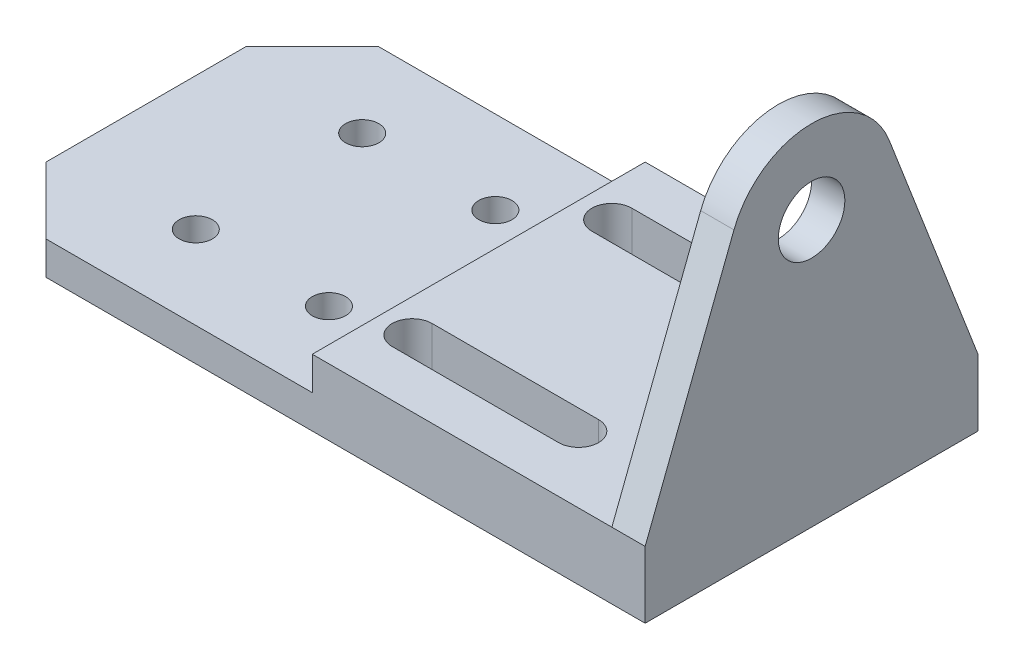
ISO-10303-21;
HEADER;
FILE_DESCRIPTION(('STEP AP214'),'2;1');
FILE_NAME('part.step','',(''),(''),'','','');
FILE_SCHEMA(('AUTOMOTIVE_DESIGN { 1 0 10303 214 1 1 1 1 }'));
ENDSEC;
DATA;
#1=APPLICATION_CONTEXT('core data for automotive mechanical design processes');
#2=APPLICATION_PROTOCOL_DEFINITION('international standard','automotive_design',2000,#1);
#3=PRODUCT_CONTEXT('',#1,'mechanical');
#4=PRODUCT('Part','Part','',(#3));
#5=PRODUCT_RELATED_PRODUCT_CATEGORY('part','',(#4));
#6=PRODUCT_DEFINITION_FORMATION('','',#4);
#7=PRODUCT_DEFINITION_CONTEXT('part definition',#1,'design');
#8=PRODUCT_DEFINITION('design','',#6,#7);
#9=PRODUCT_DEFINITION_SHAPE('','',#8);
#10=(LENGTH_UNIT() NAMED_UNIT(*) SI_UNIT(.MILLI.,.METRE.));
#11=(NAMED_UNIT(*) PLANE_ANGLE_UNIT() SI_UNIT($,.RADIAN.));
#12=(NAMED_UNIT(*) SI_UNIT($,.STERADIAN.) SOLID_ANGLE_UNIT());
#13=UNCERTAINTY_MEASURE_WITH_UNIT(LENGTH_MEASURE(1.E-05),#10,'distance_accuracy_value','');
#14=(GEOMETRIC_REPRESENTATION_CONTEXT(3) GLOBAL_UNCERTAINTY_ASSIGNED_CONTEXT((#13)) GLOBAL_UNIT_ASSIGNED_CONTEXT((#10,
#11,#12)) REPRESENTATION_CONTEXT('',''));
#15=CARTESIAN_POINT('',(0.,0.,0.));
#16=DIRECTION('',(0.,0.,1.));
#17=DIRECTION('',(1.,0.,0.));
#18=AXIS2_PLACEMENT_3D('',#15,#16,#17);
#19=CARTESIAN_POINT('',(0.,20.,100.));
#20=DIRECTION('',(1.,0.,0.));
#21=DIRECTION('',(0.,0.,-1.));
#22=AXIS2_PLACEMENT_3D('',#19,#20,#21);
#23=PLANE('',#22);
#24=DIRECTION('',(0.,0.,-1.));
#25=VECTOR('',#24,1.);
#26=CARTESIAN_POINT('',(0.,10.,100.));
#27=LINE('',#26,#25);
#28=CARTESIAN_POINT('',(0.,10.,100.));
#29=VERTEX_POINT('',#28);
#30=CARTESIAN_POINT('',(0.,10.,0.));
#31=VERTEX_POINT('',#30);
#32=EDGE_CURVE('E279',#29,#31,#27,.T.);
#33=ORIENTED_EDGE('',*,*,#32,.F.);
#34=DIRECTION('',(0.,-1.,0.));
#35=VECTOR('',#34,1.);
#36=CARTESIAN_POINT('',(0.,20.,100.));
#37=LINE('',#36,#35);
#38=CARTESIAN_POINT('',(0.,20.,100.));
#39=VERTEX_POINT('',#38);
#40=EDGE_CURVE('E295',#39,#29,#37,.T.);
#41=ORIENTED_EDGE('',*,*,#40,.F.);
#42=DIRECTION('',(0.,0.,-1.));
#43=VECTOR('',#42,1.);
#44=CARTESIAN_POINT('',(0.,20.,100.));
#45=LINE('',#44,#43);
#46=CARTESIAN_POINT('',(0.,20.,0.));
#47=VERTEX_POINT('',#46);
#48=EDGE_CURVE('E302',#39,#47,#45,.T.);
#49=ORIENTED_EDGE('',*,*,#48,.T.);
#50=DIRECTION('',(0.,-1.,0.));
#51=VECTOR('',#50,1.);
#52=CARTESIAN_POINT('',(0.,20.,0.));
#53=LINE('',#52,#51);
#54=EDGE_CURVE('E288',#47,#31,#53,.T.);
#55=ORIENTED_EDGE('',*,*,#54,.T.);
#56=EDGE_LOOP('',(#33,#41,#49,#55));
#57=FACE_BOUND('',#56,.T.);
#58=ADVANCED_FACE('F41',(#57),#23,.F.);
#59=CARTESIAN_POINT('',(0.,0.,100.));
#60=DIRECTION('',(0.,1.,0.));
#61=DIRECTION('',(0.,0.,1.));
#62=AXIS2_PLACEMENT_3D('',#59,#60,#61);
#63=PLANE('',#62);
#64=CARTESIAN_POINT('',(-60.,0.,25.));
#65=DIRECTION('',(0.,1.,0.));
#66=DIRECTION('',(0.,0.,1.));
#67=AXIS2_PLACEMENT_3D('',#64,#65,#66);
#68=CIRCLE('',#67,5.);
#69=CARTESIAN_POINT('',(-60.,0.,30.));
#70=VERTEX_POINT('',#69);
#71=EDGE_CURVE('E643',#70,#70,#68,.T.);
#72=ORIENTED_EDGE('',*,*,#71,.T.);
#73=EDGE_LOOP('',(#72));
#74=FACE_BOUND('',#73,.T.);
#75=CARTESIAN_POINT('',(-20.,0.,75.));
#76=DIRECTION('',(0.,1.,0.));
#77=DIRECTION('',(0.,0.,1.));
#78=AXIS2_PLACEMENT_3D('',#75,#76,#77);
#79=CIRCLE('',#78,5.);
#80=CARTESIAN_POINT('',(-20.,0.,80.));
#81=VERTEX_POINT('',#80);
#82=EDGE_CURVE('E644',#81,#81,#79,.T.);
#83=ORIENTED_EDGE('',*,*,#82,.T.);
#84=EDGE_LOOP('',(#83));
#85=FACE_BOUND('',#84,.T.);
#86=CARTESIAN_POINT('',(-60.,0.,75.));
#87=DIRECTION('',(0.,1.,0.));
#88=DIRECTION('',(0.,0.,1.));
#89=AXIS2_PLACEMENT_3D('',#86,#87,#88);
#90=CIRCLE('',#89,5.);
#91=CARTESIAN_POINT('',(-60.,0.,80.));
#92=VERTEX_POINT('',#91);
#93=EDGE_CURVE('E653',#92,#92,#90,.T.);
#94=ORIENTED_EDGE('',*,*,#93,.T.);
#95=EDGE_LOOP('',(#94));
#96=FACE_BOUND('',#95,.T.);
#97=CARTESIAN_POINT('',(-20.,0.,25.));
#98=DIRECTION('',(0.,1.,0.));
#99=DIRECTION('',(0.,0.,1.));
#100=AXIS2_PLACEMENT_3D('',#97,#98,#99);
#101=CIRCLE('',#100,5.);
#102=CARTESIAN_POINT('',(-20.,0.,30.));
#103=VERTEX_POINT('',#102);
#104=EDGE_CURVE('E231',#103,#103,#101,.T.);
#105=ORIENTED_EDGE('',*,*,#104,.T.);
#106=EDGE_LOOP('',(#105));
#107=FACE_BOUND('',#106,.T.);
#108=DIRECTION('',(-1.,0.,0.));
#109=VECTOR('',#108,1.);
#110=CARTESIAN_POINT('',(10.,0.,14.));
#111=LINE('',#110,#109);
#112=CARTESIAN_POINT('',(60.,0.,14.));
#113=VERTEX_POINT('',#112);
#114=CARTESIAN_POINT('',(10.,0.,14.));
#115=VERTEX_POINT('',#114);
#116=EDGE_CURVE('E184',#113,#115,#111,.T.);
#117=ORIENTED_EDGE('',*,*,#116,.T.);
#118=CARTESIAN_POINT('',(10.,0.,20.));
#119=DIRECTION('',(0.,1.,0.));
#120=DIRECTION('',(0.,0.,1.));
#121=AXIS2_PLACEMENT_3D('',#118,#119,#120);
#122=CIRCLE('',#121,6.);
#123=CARTESIAN_POINT('',(10.,0.,26.));
#124=VERTEX_POINT('',#123);
#125=EDGE_CURVE('E179',#115,#124,#122,.T.);
#126=ORIENTED_EDGE('',*,*,#125,.T.);
#127=DIRECTION('',(1.,0.,0.));
#128=VECTOR('',#127,1.);
#129=CARTESIAN_POINT('',(10.,0.,26.));
#130=LINE('',#129,#128);
#131=CARTESIAN_POINT('',(60.,0.,26.));
#132=VERTEX_POINT('',#131);
#133=EDGE_CURVE('E190',#124,#132,#130,.T.);
#134=ORIENTED_EDGE('',*,*,#133,.T.);
#135=CARTESIAN_POINT('',(60.,0.,20.));
#136=DIRECTION('',(0.,1.,0.));
#137=DIRECTION('',(0.,0.,1.));
#138=AXIS2_PLACEMENT_3D('',#135,#136,#137);
#139=CIRCLE('',#138,6.);
#140=EDGE_CURVE('E60',#132,#113,#139,.T.);
#141=ORIENTED_EDGE('',*,*,#140,.T.);
#142=EDGE_LOOP('',(#117,#126,#134,#141));
#143=FACE_BOUND('',#142,.T.);
#144=DIRECTION('',(1.,0.,0.));
#145=VECTOR('',#144,1.);
#146=CARTESIAN_POINT('',(60.,0.,86.));
#147=LINE('',#146,#145);
#148=CARTESIAN_POINT('',(10.,0.,86.));
#149=VERTEX_POINT('',#148);
#150=CARTESIAN_POINT('',(60.,0.,86.));
#151=VERTEX_POINT('',#150);
#152=EDGE_CURVE('E223',#149,#151,#147,.T.);
#153=ORIENTED_EDGE('',*,*,#152,.T.);
#154=CARTESIAN_POINT('',(60.,0.,80.));
#155=DIRECTION('',(0.,1.,0.));
#156=DIRECTION('',(0.,0.,1.));
#157=AXIS2_PLACEMENT_3D('',#154,#155,#156);
#158=CIRCLE('',#157,5.99999999999999);
#159=CARTESIAN_POINT('',(60.,0.,74.));
#160=VERTEX_POINT('',#159);
#161=EDGE_CURVE('E220',#151,#160,#158,.T.);
#162=ORIENTED_EDGE('',*,*,#161,.T.);
#163=DIRECTION('',(-1.,0.,0.));
#164=VECTOR('',#163,1.);
#165=CARTESIAN_POINT('',(60.,0.,74.));
#166=LINE('',#165,#164);
#167=CARTESIAN_POINT('',(10.,0.,74.));
#168=VERTEX_POINT('',#167);
#169=EDGE_CURVE('E219',#160,#168,#166,.T.);
#170=ORIENTED_EDGE('',*,*,#169,.T.);
#171=CARTESIAN_POINT('',(10.,0.,80.));
#172=DIRECTION('',(0.,1.,0.));
#173=DIRECTION('',(0.,0.,1.));
#174=AXIS2_PLACEMENT_3D('',#171,#172,#173);
#175=CIRCLE('',#174,5.99999999999998);
#176=EDGE_CURVE('E64',#168,#149,#175,.T.);
#177=ORIENTED_EDGE('',*,*,#176,.T.);
#178=EDGE_LOOP('',(#153,#162,#170,#177));
#179=FACE_BOUND('',#178,.T.);
#180=DIRECTION('',(1.,0.,0.));
#181=VECTOR('',#180,1.);
#182=CARTESIAN_POINT('',(0.,0.,100.));
#183=LINE('',#182,#181);
#184=CARTESIAN_POINT('',(-80.,0.,100.));
#185=VERTEX_POINT('',#184);
#186=CARTESIAN_POINT('',(100.,0.,100.));
#187=VERTEX_POINT('',#186);
#188=EDGE_CURVE('E293',#185,#187,#183,.T.);
#189=ORIENTED_EDGE('',*,*,#188,.F.);
#190=DIRECTION('',(-0.707106781186546,0.,-0.707106781186549));
#191=VECTOR('',#190,1.);
#192=CARTESIAN_POINT('',(-80.,0.,100.));
#193=LINE('',#192,#191);
#194=CARTESIAN_POINT('',(-100.,0.,79.9999999999999));
#195=VERTEX_POINT('',#194);
#196=EDGE_CURVE('E324',#185,#195,#193,.T.);
#197=ORIENTED_EDGE('',*,*,#196,.T.);
#198=DIRECTION('',(0.,0.,1.));
#199=VECTOR('',#198,1.);
#200=CARTESIAN_POINT('',(-100.,0.,0.));
#201=LINE('',#200,#199);
#202=CARTESIAN_POINT('',(-100.,0.,20.));
#203=VERTEX_POINT('',#202);
#204=EDGE_CURVE('E277',#203,#195,#201,.T.);
#205=ORIENTED_EDGE('',*,*,#204,.F.);
#206=DIRECTION('',(-0.707106781186549,0.,0.707106781186547));
#207=VECTOR('',#206,1.);
#208=CARTESIAN_POINT('',(-100.,0.,20.));
#209=LINE('',#208,#207);
#210=CARTESIAN_POINT('',(-79.9999999999999,0.,0.));
#211=VERTEX_POINT('',#210);
#212=EDGE_CURVE('E323',#203,#211,#209,.F.);
#213=ORIENTED_EDGE('',*,*,#212,.T.);
#214=DIRECTION('',(1.,0.,0.));
#215=VECTOR('',#214,1.);
#216=CARTESIAN_POINT('',(0.,0.,0.));
#217=LINE('',#216,#215);
#218=CARTESIAN_POINT('',(100.,0.,0.));
#219=VERTEX_POINT('',#218);
#220=EDGE_CURVE('E307',#211,#219,#217,.T.);
#221=ORIENTED_EDGE('',*,*,#220,.T.);
#222=DIRECTION('',(0.,0.,-1.));
#223=VECTOR('',#222,1.);
#224=CARTESIAN_POINT('',(100.,0.,100.));
#225=LINE('',#224,#223);
#226=EDGE_CURVE('E320',#187,#219,#225,.T.);
#227=ORIENTED_EDGE('',*,*,#226,.F.);
#228=EDGE_LOOP('',(#189,#197,#205,#213,#221,#227));
#229=FACE_BOUND('',#228,.T.);
#230=ADVANCED_FACE('F194',(#74,#85,#96,#107,#143,#179,#229),#63,.F.);
#231=CARTESIAN_POINT('',(100.,0.,100.));
#232=DIRECTION('',(-1.,0.,0.));
#233=DIRECTION('',(0.,0.,1.));
#234=AXIS2_PLACEMENT_3D('',#231,#232,#233);
#235=PLANE('',#234);
#236=DIRECTION('',(0.,1.,0.));
#237=VECTOR('',#236,1.);
#238=CARTESIAN_POINT('',(100.,0.,0.));
#239=LINE('',#238,#237);
#240=CARTESIAN_POINT('',(100.,20.,0.));
#241=VERTEX_POINT('',#240);
#242=EDGE_CURVE('E310',#219,#241,#239,.T.);
#243=ORIENTED_EDGE('',*,*,#242,.T.);
#244=DIRECTION('',(0.,0.932720422308954,0.360600351924129));
#245=VECTOR('',#244,1.);
#246=CARTESIAN_POINT('',(100.,20.,0.));
#247=LINE('',#246,#245);
#248=CARTESIAN_POINT('',(100.,89.0150087981032,26.6819894422761));
#249=VERTEX_POINT('',#248);
#250=EDGE_CURVE('E247',#241,#249,#247,.T.);
#251=ORIENTED_EDGE('',*,*,#250,.T.);
#252=CARTESIAN_POINT('',(100.,80.,50.));
#253=DIRECTION('',(1.,0.,0.));
#254=DIRECTION('',(0.,0.,-1.));
#255=AXIS2_PLACEMENT_3D('',#252,#253,#254);
#256=CIRCLE('',#255,25.);
#257=CARTESIAN_POINT('',(100.,89.0150087981032,73.3180105577239));
#258=VERTEX_POINT('',#257);
#259=EDGE_CURVE('E267',#249,#258,#256,.T.);
#260=ORIENTED_EDGE('',*,*,#259,.T.);
#261=DIRECTION('',(0.,-0.932720422308954,0.360600351924129));
#262=VECTOR('',#261,1.);
#263=CARTESIAN_POINT('',(100.,20.,100.));
#264=LINE('',#263,#262);
#265=CARTESIAN_POINT('',(100.,20.,100.));
#266=VERTEX_POINT('',#265);
#267=EDGE_CURVE('E260',#258,#266,#264,.T.);
#268=ORIENTED_EDGE('',*,*,#267,.T.);
#269=DIRECTION('',(0.,1.,0.));
#270=VECTOR('',#269,1.);
#271=CARTESIAN_POINT('',(100.,0.,100.));
#272=LINE('',#271,#270);
#273=EDGE_CURVE('E296',#187,#266,#272,.T.);
#274=ORIENTED_EDGE('',*,*,#273,.F.);
#275=ORIENTED_EDGE('',*,*,#226,.T.);
#276=EDGE_LOOP('',(#243,#251,#260,#268,#274,#275));
#277=FACE_BOUND('',#276,.T.);
#278=CARTESIAN_POINT('',(100.,80.,50.));
#279=DIRECTION('',(1.,0.,0.));
#280=DIRECTION('',(0.,0.,-1.));
#281=AXIS2_PLACEMENT_3D('',#278,#279,#280);
#282=CIRCLE('',#281,10.);
#283=CARTESIAN_POINT('',(100.,80.,40.));
#284=VERTEX_POINT('',#283);
#285=EDGE_CURVE('E213',#284,#284,#282,.T.);
#286=ORIENTED_EDGE('',*,*,#285,.F.);
#287=EDGE_LOOP('',(#286));
#288=FACE_BOUND('',#287,.T.);
#289=ADVANCED_FACE('F365',(#277,#288),#235,.F.);
#290=CARTESIAN_POINT('',(100.,20.,100.));
#291=DIRECTION('',(0.,-1.,0.));
#292=DIRECTION('',(0.,0.,-1.));
#293=AXIS2_PLACEMENT_3D('',#290,#291,#292);
#294=PLANE('',#293);
#295=DIRECTION('',(1.,0.,0.));
#296=VECTOR('',#295,1.);
#297=CARTESIAN_POINT('',(10.,20.,26.));
#298=LINE('',#297,#296);
#299=CARTESIAN_POINT('',(10.,20.,26.));
#300=VERTEX_POINT('',#299);
#301=CARTESIAN_POINT('',(60.,20.,26.));
#302=VERTEX_POINT('',#301);
#303=EDGE_CURVE('E206',#300,#302,#298,.T.);
#304=ORIENTED_EDGE('',*,*,#303,.F.);
#305=CARTESIAN_POINT('',(10.,20.,20.));
#306=DIRECTION('',(0.,1.,0.));
#307=DIRECTION('',(0.,0.,1.));
#308=AXIS2_PLACEMENT_3D('',#305,#306,#307);
#309=CIRCLE('',#308,6.);
#310=CARTESIAN_POINT('',(10.,20.,14.));
#311=VERTEX_POINT('',#310);
#312=EDGE_CURVE('E178',#311,#300,#309,.T.);
#313=ORIENTED_EDGE('',*,*,#312,.F.);
#314=DIRECTION('',(-1.,0.,0.));
#315=VECTOR('',#314,1.);
#316=CARTESIAN_POINT('',(10.,20.,14.));
#317=LINE('',#316,#315);
#318=CARTESIAN_POINT('',(60.,20.,14.));
#319=VERTEX_POINT('',#318);
#320=EDGE_CURVE('E193',#319,#311,#317,.T.);
#321=ORIENTED_EDGE('',*,*,#320,.F.);
#322=CARTESIAN_POINT('',(60.,20.,20.));
#323=DIRECTION('',(0.,1.,0.));
#324=DIRECTION('',(0.,0.,1.));
#325=AXIS2_PLACEMENT_3D('',#322,#323,#324);
#326=CIRCLE('',#325,6.);
#327=EDGE_CURVE('E197',#302,#319,#326,.T.);
#328=ORIENTED_EDGE('',*,*,#327,.F.);
#329=EDGE_LOOP('',(#304,#313,#321,#328));
#330=FACE_BOUND('',#329,.T.);
#331=DIRECTION('',(-1.,0.,0.));
#332=VECTOR('',#331,1.);
#333=CARTESIAN_POINT('',(60.,20.,74.));
#334=LINE('',#333,#332);
#335=CARTESIAN_POINT('',(60.,20.,74.));
#336=VERTEX_POINT('',#335);
#337=CARTESIAN_POINT('',(10.,20.,74.));
#338=VERTEX_POINT('',#337);
#339=EDGE_CURVE('E234',#336,#338,#334,.T.);
#340=ORIENTED_EDGE('',*,*,#339,.F.);
#341=CARTESIAN_POINT('',(60.,20.,80.));
#342=DIRECTION('',(0.,1.,0.));
#343=DIRECTION('',(0.,0.,1.));
#344=AXIS2_PLACEMENT_3D('',#341,#342,#343);
#345=CIRCLE('',#344,5.99999999999999);
#346=CARTESIAN_POINT('',(60.,20.,86.));
#347=VERTEX_POINT('',#346);
#348=EDGE_CURVE('E227',#347,#336,#345,.T.);
#349=ORIENTED_EDGE('',*,*,#348,.F.);
#350=DIRECTION('',(1.,0.,0.));
#351=VECTOR('',#350,1.);
#352=CARTESIAN_POINT('',(60.,20.,86.));
#353=LINE('',#352,#351);
#354=CARTESIAN_POINT('',(10.,20.,86.));
#355=VERTEX_POINT('',#354);
#356=EDGE_CURVE('E222',#355,#347,#353,.T.);
#357=ORIENTED_EDGE('',*,*,#356,.F.);
#358=CARTESIAN_POINT('',(10.,20.,80.));
#359=DIRECTION('',(0.,1.,0.));
#360=DIRECTION('',(0.,0.,1.));
#361=AXIS2_PLACEMENT_3D('',#358,#359,#360);
#362=CIRCLE('',#361,5.99999999999998);
#363=EDGE_CURVE('E232',#338,#355,#362,.T.);
#364=ORIENTED_EDGE('',*,*,#363,.F.);
#365=EDGE_LOOP('',(#340,#349,#357,#364));
#366=FACE_BOUND('',#365,.T.);
#367=DIRECTION('',(-1.,0.,0.));
#368=VECTOR('',#367,1.);
#369=CARTESIAN_POINT('',(100.,20.,100.));
#370=LINE('',#369,#368);
#371=CARTESIAN_POINT('',(90.,20.,100.));
#372=VERTEX_POINT('',#371);
#373=EDGE_CURVE('E304',#372,#39,#370,.T.);
#374=ORIENTED_EDGE('',*,*,#373,.F.);
#375=DIRECTION('',(0.,0.,-1.));
#376=VECTOR('',#375,1.);
#377=CARTESIAN_POINT('',(90.,20.,100.));
#378=LINE('',#377,#376);
#379=CARTESIAN_POINT('',(90.,20.,0.));
#380=VERTEX_POINT('',#379);
#381=EDGE_CURVE('E251',#372,#380,#378,.T.);
#382=ORIENTED_EDGE('',*,*,#381,.T.);
#383=DIRECTION('',(-1.,0.,0.));
#384=VECTOR('',#383,1.);
#385=CARTESIAN_POINT('',(100.,20.,0.));
#386=LINE('',#385,#384);
#387=EDGE_CURVE('E315',#380,#47,#386,.T.);
#388=ORIENTED_EDGE('',*,*,#387,.T.);
#389=ORIENTED_EDGE('',*,*,#48,.F.);
#390=EDGE_LOOP('',(#374,#382,#388,#389));
#391=FACE_BOUND('',#390,.T.);
#392=ADVANCED_FACE('F376',(#330,#366,#391),#294,.F.);
#393=CARTESIAN_POINT('',(0.,0.,100.));
#394=DIRECTION('',(0.,0.,1.));
#395=DIRECTION('',(1.,0.,0.));
#396=AXIS2_PLACEMENT_3D('',#393,#394,#395);
#397=PLANE('',#396);
#398=DIRECTION('',(1.,0.,0.));
#399=VECTOR('',#398,1.);
#400=CARTESIAN_POINT('',(-100.,10.,100.));
#401=LINE('',#400,#399);
#402=CARTESIAN_POINT('',(-80.,10.,100.));
#403=VERTEX_POINT('',#402);
#404=EDGE_CURVE('E286',#403,#29,#401,.T.);
#405=ORIENTED_EDGE('',*,*,#404,.F.);
#406=DIRECTION('',(0.,-1.,0.));
#407=VECTOR('',#406,1.);
#408=CARTESIAN_POINT('',(-80.,0.,100.));
#409=LINE('',#408,#407);
#410=EDGE_CURVE('E319',#403,#185,#409,.T.);
#411=ORIENTED_EDGE('',*,*,#410,.T.);
#412=ORIENTED_EDGE('',*,*,#188,.T.);
#413=ORIENTED_EDGE('',*,*,#273,.T.);
#414=EDGE_CURVE('E301',#266,#372,#370,.T.);
#415=ORIENTED_EDGE('',*,*,#414,.T.);
#416=ORIENTED_EDGE('',*,*,#373,.T.);
#417=ORIENTED_EDGE('',*,*,#40,.T.);
#418=EDGE_LOOP('',(#405,#411,#412,#413,#415,#416,#417));
#419=FACE_BOUND('',#418,.T.);
#420=ADVANCED_FACE('F345',(#419),#397,.T.);
#421=CARTESIAN_POINT('',(0.,0.,0.));
#422=DIRECTION('',(0.,0.,1.));
#423=DIRECTION('',(1.,0.,0.));
#424=AXIS2_PLACEMENT_3D('',#421,#422,#423);
#425=PLANE('',#424);
#426=ORIENTED_EDGE('',*,*,#220,.F.);
#427=DIRECTION('',(0.,1.,0.));
#428=VECTOR('',#427,1.);
#429=CARTESIAN_POINT('',(-79.9999999999999,0.,0.));
#430=LINE('',#429,#428);
#431=CARTESIAN_POINT('',(-79.9999999999999,10.,0.));
#432=VERTEX_POINT('',#431);
#433=EDGE_CURVE('E11',#211,#432,#430,.T.);
#434=ORIENTED_EDGE('',*,*,#433,.T.);
#435=DIRECTION('',(-1.,0.,0.));
#436=VECTOR('',#435,1.);
#437=CARTESIAN_POINT('',(0.,10.,0.));
#438=LINE('',#437,#436);
#439=EDGE_CURVE('E283',#31,#432,#438,.T.);
#440=ORIENTED_EDGE('',*,*,#439,.F.);
#441=ORIENTED_EDGE('',*,*,#54,.F.);
#442=ORIENTED_EDGE('',*,*,#387,.F.);
#443=EDGE_CURVE('E298',#241,#380,#386,.T.);
#444=ORIENTED_EDGE('',*,*,#443,.F.);
#445=ORIENTED_EDGE('',*,*,#242,.F.);
#446=EDGE_LOOP('',(#426,#434,#440,#441,#442,#444,#445));
#447=FACE_BOUND('',#446,.T.);
#448=ADVANCED_FACE('F358',(#447),#425,.F.);
#449=CARTESIAN_POINT('',(-100.,10.,0.));
#450=DIRECTION('',(1.,0.,0.));
#451=DIRECTION('',(0.,0.,-1.));
#452=AXIS2_PLACEMENT_3D('',#449,#450,#451);
#453=PLANE('',#452);
#454=ORIENTED_EDGE('',*,*,#204,.T.);
#455=DIRECTION('',(0.,1.,0.));
#456=VECTOR('',#455,1.);
#457=CARTESIAN_POINT('',(-100.,10.,79.9999999999999));
#458=LINE('',#457,#456);
#459=CARTESIAN_POINT('',(-100.,10.,79.9999999999999));
#460=VERTEX_POINT('',#459);
#461=EDGE_CURVE('E329',#195,#460,#458,.T.);
#462=ORIENTED_EDGE('',*,*,#461,.T.);
#463=DIRECTION('',(0.,0.,1.));
#464=VECTOR('',#463,1.);
#465=CARTESIAN_POINT('',(-100.,10.,0.));
#466=LINE('',#465,#464);
#467=CARTESIAN_POINT('',(-100.,10.,20.));
#468=VERTEX_POINT('',#467);
#469=EDGE_CURVE('E282',#468,#460,#466,.T.);
#470=ORIENTED_EDGE('',*,*,#469,.F.);
#471=DIRECTION('',(0.,-1.,0.));
#472=VECTOR('',#471,1.);
#473=CARTESIAN_POINT('',(-100.,10.,20.));
#474=LINE('',#473,#472);
#475=EDGE_CURVE('E330',#468,#203,#474,.T.);
#476=ORIENTED_EDGE('',*,*,#475,.T.);
#477=EDGE_LOOP('',(#454,#462,#470,#476));
#478=FACE_BOUND('',#477,.T.);
#479=ADVANCED_FACE('F353',(#478),#453,.F.);
#480=CARTESIAN_POINT('',(0.,10.,0.));
#481=DIRECTION('',(0.,1.,0.));
#482=DIRECTION('',(0.,0.,1.));
#483=AXIS2_PLACEMENT_3D('',#480,#481,#482);
#484=PLANE('',#483);
#485=CARTESIAN_POINT('',(-60.,10.,25.));
#486=DIRECTION('',(0.,1.,0.));
#487=DIRECTION('',(0.,0.,1.));
#488=AXIS2_PLACEMENT_3D('',#485,#486,#487);
#489=CIRCLE('',#488,5.);
#490=CARTESIAN_POINT('',(-60.,10.,30.));
#491=VERTEX_POINT('',#490);
#492=EDGE_CURVE('E641',#491,#491,#489,.T.);
#493=ORIENTED_EDGE('',*,*,#492,.F.);
#494=EDGE_LOOP('',(#493));
#495=FACE_BOUND('',#494,.T.);
#496=CARTESIAN_POINT('',(-20.,10.,75.));
#497=DIRECTION('',(0.,1.,0.));
#498=DIRECTION('',(0.,0.,1.));
#499=AXIS2_PLACEMENT_3D('',#496,#497,#498);
#500=CIRCLE('',#499,5.);
#501=CARTESIAN_POINT('',(-20.,10.,80.));
#502=VERTEX_POINT('',#501);
#503=EDGE_CURVE('E648',#502,#502,#500,.T.);
#504=ORIENTED_EDGE('',*,*,#503,.F.);
#505=EDGE_LOOP('',(#504));
#506=FACE_BOUND('',#505,.T.);
#507=CARTESIAN_POINT('',(-60.,10.,75.));
#508=DIRECTION('',(0.,1.,0.));
#509=DIRECTION('',(0.,0.,1.));
#510=AXIS2_PLACEMENT_3D('',#507,#508,#509);
#511=CIRCLE('',#510,5.);
#512=CARTESIAN_POINT('',(-60.,10.,80.));
#513=VERTEX_POINT('',#512);
#514=EDGE_CURVE('E661',#513,#513,#511,.T.);
#515=ORIENTED_EDGE('',*,*,#514,.F.);
#516=EDGE_LOOP('',(#515));
#517=FACE_BOUND('',#516,.T.);
#518=CARTESIAN_POINT('',(-20.,10.,25.));
#519=DIRECTION('',(0.,1.,0.));
#520=DIRECTION('',(0.,0.,1.));
#521=AXIS2_PLACEMENT_3D('',#518,#519,#520);
#522=CIRCLE('',#521,5.);
#523=CARTESIAN_POINT('',(-20.,10.,30.));
#524=VERTEX_POINT('',#523);
#525=EDGE_CURVE('E199',#524,#524,#522,.T.);
#526=ORIENTED_EDGE('',*,*,#525,.F.);
#527=EDGE_LOOP('',(#526));
#528=FACE_BOUND('',#527,.T.);
#529=ORIENTED_EDGE('',*,*,#469,.T.);
#530=DIRECTION('',(0.707106781186546,0.,0.707106781186549));
#531=VECTOR('',#530,1.);
#532=CARTESIAN_POINT('',(-90.0000000000002,10.,89.9999999999998));
#533=LINE('',#532,#531);
#534=EDGE_CURVE('E49',#460,#403,#533,.T.);
#535=ORIENTED_EDGE('',*,*,#534,.T.);
#536=ORIENTED_EDGE('',*,*,#404,.T.);
#537=ORIENTED_EDGE('',*,*,#32,.T.);
#538=ORIENTED_EDGE('',*,*,#439,.T.);
#539=DIRECTION('',(0.707106781186549,0.,-0.707106781186547));
#540=VECTOR('',#539,1.);
#541=CARTESIAN_POINT('',(-39.9999999999999,10.,-40.));
#542=LINE('',#541,#540);
#543=EDGE_CURVE('E335',#432,#468,#542,.F.);
#544=ORIENTED_EDGE('',*,*,#543,.T.);
#545=EDGE_LOOP('',(#529,#535,#536,#537,#538,#544));
#546=FACE_BOUND('',#545,.T.);
#547=ADVANCED_FACE('F338',(#495,#506,#517,#528,#546),#484,.T.);
#548=CARTESIAN_POINT('',(-80.,0.,100.));
#549=DIRECTION('',(-0.707106781186549,0.,0.707106781186546));
#550=DIRECTION('',(0.,1.,0.));
#551=AXIS2_PLACEMENT_3D('',#548,#549,#550);
#552=PLANE('',#551);
#553=ORIENTED_EDGE('',*,*,#534,.F.);
#554=ORIENTED_EDGE('',*,*,#461,.F.);
#555=ORIENTED_EDGE('',*,*,#196,.F.);
#556=ORIENTED_EDGE('',*,*,#410,.F.);
#557=EDGE_LOOP('',(#553,#554,#555,#556));
#558=FACE_BOUND('',#557,.T.);
#559=ADVANCED_FACE('F347',(#558),#552,.T.);
#560=CARTESIAN_POINT('',(-100.,10.,20.));
#561=DIRECTION('',(0.707106781186547,0.,0.707106781186549));
#562=DIRECTION('',(0.,-1.,0.));
#563=AXIS2_PLACEMENT_3D('',#560,#561,#562);
#564=PLANE('',#563);
#565=ORIENTED_EDGE('',*,*,#543,.F.);
#566=ORIENTED_EDGE('',*,*,#433,.F.);
#567=ORIENTED_EDGE('',*,*,#212,.F.);
#568=ORIENTED_EDGE('',*,*,#475,.F.);
#569=EDGE_LOOP('',(#565,#566,#567,#568));
#570=FACE_BOUND('',#569,.T.);
#571=ADVANCED_FACE('F42',(#570),#564,.F.);
#572=CARTESIAN_POINT('',(90.,20.,100.));
#573=DIRECTION('',(0.,0.360600351924129,0.932720422308955));
#574=DIRECTION('',(0.,-0.932720422308955,0.360600351924129));
#575=AXIS2_PLACEMENT_3D('',#572,#573,#574);
#576=PLANE('',#575);
#577=ORIENTED_EDGE('',*,*,#267,.F.);
#578=DIRECTION('',(1.,0.,0.));
#579=VECTOR('',#578,1.);
#580=CARTESIAN_POINT('',(90.,89.0150087981032,73.3180105577239));
#581=LINE('',#580,#579);
#582=CARTESIAN_POINT('',(90.,89.0150087981032,73.3180105577239));
#583=VERTEX_POINT('',#582);
#584=EDGE_CURVE('E273',#583,#258,#581,.T.);
#585=ORIENTED_EDGE('',*,*,#584,.F.);
#586=DIRECTION('',(0.,-0.932720422308954,0.360600351924129));
#587=VECTOR('',#586,1.);
#588=CARTESIAN_POINT('',(90.,20.,100.));
#589=LINE('',#588,#587);
#590=EDGE_CURVE('E263',#583,#372,#589,.T.);
#591=ORIENTED_EDGE('',*,*,#590,.T.);
#592=ORIENTED_EDGE('',*,*,#414,.F.);
#593=EDGE_LOOP('',(#577,#585,#591,#592));
#594=FACE_BOUND('',#593,.T.);
#595=ADVANCED_FACE('F371',(#594),#576,.T.);
#596=CARTESIAN_POINT('',(90.,80.,50.));
#597=DIRECTION('',(1.,0.,0.));
#598=DIRECTION('',(0.,0.,-1.));
#599=AXIS2_PLACEMENT_3D('',#596,#597,#598);
#600=CYLINDRICAL_SURFACE('',#599,25.);
#601=ORIENTED_EDGE('',*,*,#259,.F.);
#602=DIRECTION('',(1.,0.,0.));
#603=VECTOR('',#602,1.);
#604=CARTESIAN_POINT('',(90.,89.0150087981032,26.6819894422761));
#605=LINE('',#604,#603);
#606=CARTESIAN_POINT('',(90.,89.0150087981032,26.6819894422761));
#607=VERTEX_POINT('',#606);
#608=EDGE_CURVE('E266',#607,#249,#605,.T.);
#609=ORIENTED_EDGE('',*,*,#608,.F.);
#610=CARTESIAN_POINT('',(90.,80.,50.));
#611=DIRECTION('',(1.,0.,0.));
#612=DIRECTION('',(0.,0.,-1.));
#613=AXIS2_PLACEMENT_3D('',#610,#611,#612);
#614=CIRCLE('',#613,25.);
#615=EDGE_CURVE('E257',#607,#583,#614,.T.);
#616=ORIENTED_EDGE('',*,*,#615,.T.);
#617=ORIENTED_EDGE('',*,*,#584,.T.);
#618=EDGE_LOOP('',(#601,#609,#616,#617));
#619=FACE_BOUND('',#618,.T.);
#620=ADVANCED_FACE('F437',(#619),#600,.T.);
#621=CARTESIAN_POINT('',(90.,20.,0.));
#622=DIRECTION('',(0.,0.360600351924129,-0.932720422308955));
#623=DIRECTION('',(0.,0.932720422308955,0.360600351924129));
#624=AXIS2_PLACEMENT_3D('',#621,#622,#623);
#625=PLANE('',#624);
#626=ORIENTED_EDGE('',*,*,#250,.F.);
#627=ORIENTED_EDGE('',*,*,#443,.T.);
#628=DIRECTION('',(0.,0.932720422308954,0.360600351924129));
#629=VECTOR('',#628,1.);
#630=CARTESIAN_POINT('',(90.,20.,0.));
#631=LINE('',#630,#629);
#632=EDGE_CURVE('E258',#380,#607,#631,.T.);
#633=ORIENTED_EDGE('',*,*,#632,.T.);
#634=ORIENTED_EDGE('',*,*,#608,.T.);
#635=EDGE_LOOP('',(#626,#627,#633,#634));
#636=FACE_BOUND('',#635,.T.);
#637=ADVANCED_FACE('F403',(#636),#625,.T.);
#638=CARTESIAN_POINT('',(90.,80.,50.));
#639=DIRECTION('',(1.,0.,0.));
#640=DIRECTION('',(0.,0.,-1.));
#641=AXIS2_PLACEMENT_3D('',#638,#639,#640);
#642=PLANE('',#641);
#643=CARTESIAN_POINT('',(90.,80.,50.));
#644=DIRECTION('',(1.,0.,0.));
#645=DIRECTION('',(0.,0.,-1.));
#646=AXIS2_PLACEMENT_3D('',#643,#644,#645);
#647=CIRCLE('',#646,10.);
#648=CARTESIAN_POINT('',(90.,80.,40.));
#649=VERTEX_POINT('',#648);
#650=EDGE_CURVE('E246',#649,#649,#647,.T.);
#651=ORIENTED_EDGE('',*,*,#650,.T.);
#652=EDGE_LOOP('',(#651));
#653=FACE_BOUND('',#652,.T.);
#654=ORIENTED_EDGE('',*,*,#381,.F.);
#655=ORIENTED_EDGE('',*,*,#590,.F.);
#656=ORIENTED_EDGE('',*,*,#615,.F.);
#657=ORIENTED_EDGE('',*,*,#632,.F.);
#658=EDGE_LOOP('',(#654,#655,#656,#657));
#659=FACE_BOUND('',#658,.T.);
#660=ADVANCED_FACE('F455',(#653,#659),#642,.F.);
#661=CARTESIAN_POINT('',(90.,80.,50.));
#662=DIRECTION('',(1.,0.,0.));
#663=DIRECTION('',(0.,0.,-1.));
#664=AXIS2_PLACEMENT_3D('',#661,#662,#663);
#665=CYLINDRICAL_SURFACE('',#664,10.);
#666=ORIENTED_EDGE('',*,*,#650,.F.);
#667=EDGE_LOOP('',(#666));
#668=FACE_BOUND('',#667,.T.);
#669=ORIENTED_EDGE('',*,*,#285,.T.);
#670=EDGE_LOOP('',(#669));
#671=FACE_BOUND('',#670,.T.);
#672=ADVANCED_FACE('F463',(#668,#671),#665,.F.);
#673=CARTESIAN_POINT('',(60.,0.,80.));
#674=DIRECTION('',(0.,1.,0.));
#675=DIRECTION('',(0.,0.,1.));
#676=AXIS2_PLACEMENT_3D('',#673,#674,#675);
#677=CYLINDRICAL_SURFACE('',#676,5.99999999999999);
#678=ORIENTED_EDGE('',*,*,#348,.T.);
#679=DIRECTION('',(0.,1.,0.));
#680=VECTOR('',#679,1.);
#681=CARTESIAN_POINT('',(60.,0.,74.));
#682=LINE('',#681,#680);
#683=EDGE_CURVE('E226',#160,#336,#682,.T.);
#684=ORIENTED_EDGE('',*,*,#683,.F.);
#685=ORIENTED_EDGE('',*,*,#161,.F.);
#686=DIRECTION('',(0.,1.,0.));
#687=VECTOR('',#686,1.);
#688=CARTESIAN_POINT('',(60.,0.,86.));
#689=LINE('',#688,#687);
#690=EDGE_CURVE('E210',#151,#347,#689,.T.);
#691=ORIENTED_EDGE('',*,*,#690,.T.);
#692=EDGE_LOOP('',(#678,#684,#685,#691));
#693=FACE_BOUND('',#692,.T.);
#694=ADVANCED_FACE('F468',(#693),#677,.F.);
#695=CARTESIAN_POINT('',(60.,0.,86.));
#696=DIRECTION('',(0.,0.,1.));
#697=DIRECTION('',(1.,0.,0.));
#698=AXIS2_PLACEMENT_3D('',#695,#696,#697);
#699=PLANE('',#698);
#700=ORIENTED_EDGE('',*,*,#356,.T.);
#701=ORIENTED_EDGE('',*,*,#690,.F.);
#702=ORIENTED_EDGE('',*,*,#152,.F.);
#703=DIRECTION('',(0.,1.,0.));
#704=VECTOR('',#703,1.);
#705=CARTESIAN_POINT('',(10.,0.,86.));
#706=LINE('',#705,#704);
#707=EDGE_CURVE('E243',#149,#355,#706,.T.);
#708=ORIENTED_EDGE('',*,*,#707,.T.);
#709=EDGE_LOOP('',(#700,#701,#702,#708));
#710=FACE_BOUND('',#709,.T.);
#711=ADVANCED_FACE('F482',(#710),#699,.F.);
#712=CARTESIAN_POINT('',(10.,0.,80.));
#713=DIRECTION('',(0.,1.,0.));
#714=DIRECTION('',(0.,0.,1.));
#715=AXIS2_PLACEMENT_3D('',#712,#713,#714);
#716=CYLINDRICAL_SURFACE('',#715,5.99999999999998);
#717=ORIENTED_EDGE('',*,*,#363,.T.);
#718=ORIENTED_EDGE('',*,*,#707,.F.);
#719=ORIENTED_EDGE('',*,*,#176,.F.);
#720=DIRECTION('',(0.,1.,0.));
#721=VECTOR('',#720,1.);
#722=CARTESIAN_POINT('',(10.,0.,74.));
#723=LINE('',#722,#721);
#724=EDGE_CURVE('E241',#168,#338,#723,.T.);
#725=ORIENTED_EDGE('',*,*,#724,.T.);
#726=EDGE_LOOP('',(#717,#718,#719,#725));
#727=FACE_BOUND('',#726,.T.);
#728=ADVANCED_FACE('F492',(#727),#716,.F.);
#729=CARTESIAN_POINT('',(60.,0.,74.));
#730=DIRECTION('',(0.,0.,-1.));
#731=DIRECTION('',(-1.,0.,0.));
#732=AXIS2_PLACEMENT_3D('',#729,#730,#731);
#733=PLANE('',#732);
#734=ORIENTED_EDGE('',*,*,#339,.T.);
#735=ORIENTED_EDGE('',*,*,#724,.F.);
#736=ORIENTED_EDGE('',*,*,#169,.F.);
#737=ORIENTED_EDGE('',*,*,#683,.T.);
#738=EDGE_LOOP('',(#734,#735,#736,#737));
#739=FACE_BOUND('',#738,.T.);
#740=ADVANCED_FACE('F505',(#739),#733,.F.);
#741=CARTESIAN_POINT('',(10.,0.,20.));
#742=DIRECTION('',(0.,1.,0.));
#743=DIRECTION('',(0.,0.,1.));
#744=AXIS2_PLACEMENT_3D('',#741,#742,#743);
#745=CYLINDRICAL_SURFACE('',#744,6.);
#746=ORIENTED_EDGE('',*,*,#312,.T.);
#747=DIRECTION('',(0.,1.,0.));
#748=VECTOR('',#747,1.);
#749=CARTESIAN_POINT('',(10.,0.,26.));
#750=LINE('',#749,#748);
#751=EDGE_CURVE('E175',#124,#300,#750,.T.);
#752=ORIENTED_EDGE('',*,*,#751,.F.);
#753=ORIENTED_EDGE('',*,*,#125,.F.);
#754=DIRECTION('',(0.,1.,0.));
#755=VECTOR('',#754,1.);
#756=CARTESIAN_POINT('',(10.,0.,14.));
#757=LINE('',#756,#755);
#758=EDGE_CURVE('E211',#115,#311,#757,.T.);
#759=ORIENTED_EDGE('',*,*,#758,.T.);
#760=EDGE_LOOP('',(#746,#752,#753,#759));
#761=FACE_BOUND('',#760,.T.);
#762=ADVANCED_FACE('F172',(#761),#745,.F.);
#763=CARTESIAN_POINT('',(10.,0.,14.));
#764=DIRECTION('',(0.,0.,-1.));
#765=DIRECTION('',(-1.,0.,0.));
#766=AXIS2_PLACEMENT_3D('',#763,#764,#765);
#767=PLANE('',#766);
#768=ORIENTED_EDGE('',*,*,#320,.T.);
#769=ORIENTED_EDGE('',*,*,#758,.F.);
#770=ORIENTED_EDGE('',*,*,#116,.F.);
#771=DIRECTION('',(0.,1.,0.));
#772=VECTOR('',#771,1.);
#773=CARTESIAN_POINT('',(60.,0.,14.));
#774=LINE('',#773,#772);
#775=EDGE_CURVE('E212',#113,#319,#774,.T.);
#776=ORIENTED_EDGE('',*,*,#775,.T.);
#777=EDGE_LOOP('',(#768,#769,#770,#776));
#778=FACE_BOUND('',#777,.T.);
#779=ADVANCED_FACE('F516',(#778),#767,.F.);
#780=CARTESIAN_POINT('',(60.,0.,20.));
#781=DIRECTION('',(0.,1.,0.));
#782=DIRECTION('',(0.,0.,1.));
#783=AXIS2_PLACEMENT_3D('',#780,#781,#782);
#784=CYLINDRICAL_SURFACE('',#783,6.);
#785=ORIENTED_EDGE('',*,*,#327,.T.);
#786=ORIENTED_EDGE('',*,*,#775,.F.);
#787=ORIENTED_EDGE('',*,*,#140,.F.);
#788=DIRECTION('',(0.,1.,0.));
#789=VECTOR('',#788,1.);
#790=CARTESIAN_POINT('',(60.,0.,26.));
#791=LINE('',#790,#789);
#792=EDGE_CURVE('E181',#132,#302,#791,.T.);
#793=ORIENTED_EDGE('',*,*,#792,.T.);
#794=EDGE_LOOP('',(#785,#786,#787,#793));
#795=FACE_BOUND('',#794,.T.);
#796=ADVANCED_FACE('F528',(#795),#784,.F.);
#797=CARTESIAN_POINT('',(10.,0.,26.));
#798=DIRECTION('',(0.,0.,1.));
#799=DIRECTION('',(1.,0.,0.));
#800=AXIS2_PLACEMENT_3D('',#797,#798,#799);
#801=PLANE('',#800);
#802=ORIENTED_EDGE('',*,*,#303,.T.);
#803=ORIENTED_EDGE('',*,*,#792,.F.);
#804=ORIENTED_EDGE('',*,*,#133,.F.);
#805=ORIENTED_EDGE('',*,*,#751,.T.);
#806=EDGE_LOOP('',(#802,#803,#804,#805));
#807=FACE_BOUND('',#806,.T.);
#808=ADVANCED_FACE('F186',(#807),#801,.F.);
#809=CARTESIAN_POINT('',(-20.,0.,25.));
#810=DIRECTION('',(0.,1.,0.));
#811=DIRECTION('',(0.,0.,1.));
#812=AXIS2_PLACEMENT_3D('',#809,#810,#811);
#813=CYLINDRICAL_SURFACE('',#812,5.);
#814=ORIENTED_EDGE('',*,*,#104,.F.);
#815=EDGE_LOOP('',(#814));
#816=FACE_BOUND('',#815,.T.);
#817=ORIENTED_EDGE('',*,*,#525,.T.);
#818=EDGE_LOOP('',(#817));
#819=FACE_BOUND('',#818,.T.);
#820=ADVANCED_FACE('F541',(#816,#819),#813,.F.);
#821=CARTESIAN_POINT('',(-60.,0.,75.));
#822=DIRECTION('',(0.,1.,0.));
#823=DIRECTION('',(0.,0.,1.));
#824=AXIS2_PLACEMENT_3D('',#821,#822,#823);
#825=CYLINDRICAL_SURFACE('',#824,5.);
#826=ORIENTED_EDGE('',*,*,#93,.F.);
#827=EDGE_LOOP('',(#826));
#828=FACE_BOUND('',#827,.T.);
#829=ORIENTED_EDGE('',*,*,#514,.T.);
#830=EDGE_LOOP('',(#829));
#831=FACE_BOUND('',#830,.T.);
#832=ADVANCED_FACE('F603',(#828,#831),#825,.F.);
#833=CARTESIAN_POINT('',(-20.,0.,75.));
#834=DIRECTION('',(0.,1.,0.));
#835=DIRECTION('',(0.,0.,1.));
#836=AXIS2_PLACEMENT_3D('',#833,#834,#835);
#837=CYLINDRICAL_SURFACE('',#836,5.);
#838=ORIENTED_EDGE('',*,*,#82,.F.);
#839=EDGE_LOOP('',(#838));
#840=FACE_BOUND('',#839,.T.);
#841=ORIENTED_EDGE('',*,*,#503,.T.);
#842=EDGE_LOOP('',(#841));
#843=FACE_BOUND('',#842,.T.);
#844=ADVANCED_FACE('F611',(#840,#843),#837,.F.);
#845=CARTESIAN_POINT('',(-60.,0.,25.));
#846=DIRECTION('',(0.,1.,0.));
#847=DIRECTION('',(0.,0.,1.));
#848=AXIS2_PLACEMENT_3D('',#845,#846,#847);
#849=CYLINDRICAL_SURFACE('',#848,5.);
#850=ORIENTED_EDGE('',*,*,#71,.F.);
#851=EDGE_LOOP('',(#850));
#852=FACE_BOUND('',#851,.T.);
#853=ORIENTED_EDGE('',*,*,#492,.T.);
#854=EDGE_LOOP('',(#853));
#855=FACE_BOUND('',#854,.T.);
#856=ADVANCED_FACE('F625',(#852,#855),#849,.F.);
#857=CLOSED_SHELL('',(#58,#230,#289,#392,#420,#448,#479,#547,#559,#571,#595,#620,#637,#660,#672,
#694,#711,#728,#740,#762,#779,#796,#808,#820,#832,#844,#856));
#858=MANIFOLD_SOLID_BREP('B2',#857);
#859=ADVANCED_BREP_SHAPE_REPRESENTATION('',(#18,#858),#14);
#860=SHAPE_DEFINITION_REPRESENTATION(#9,#859);
ENDSEC;
END-ISO-10303-21;
